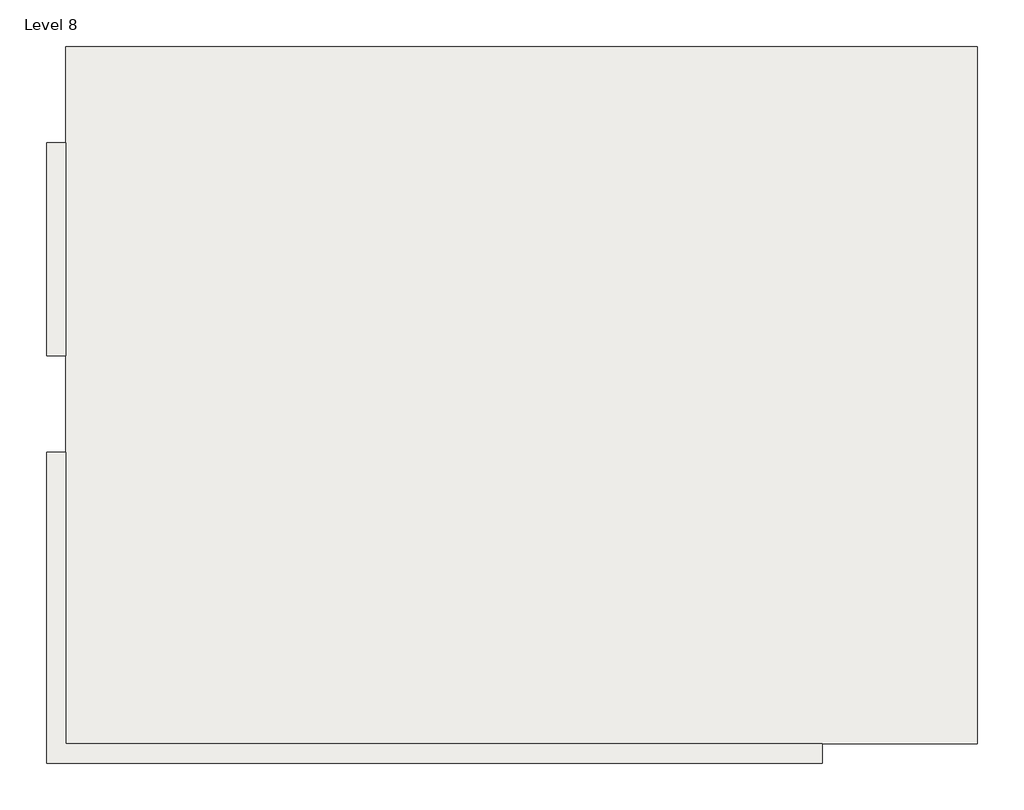
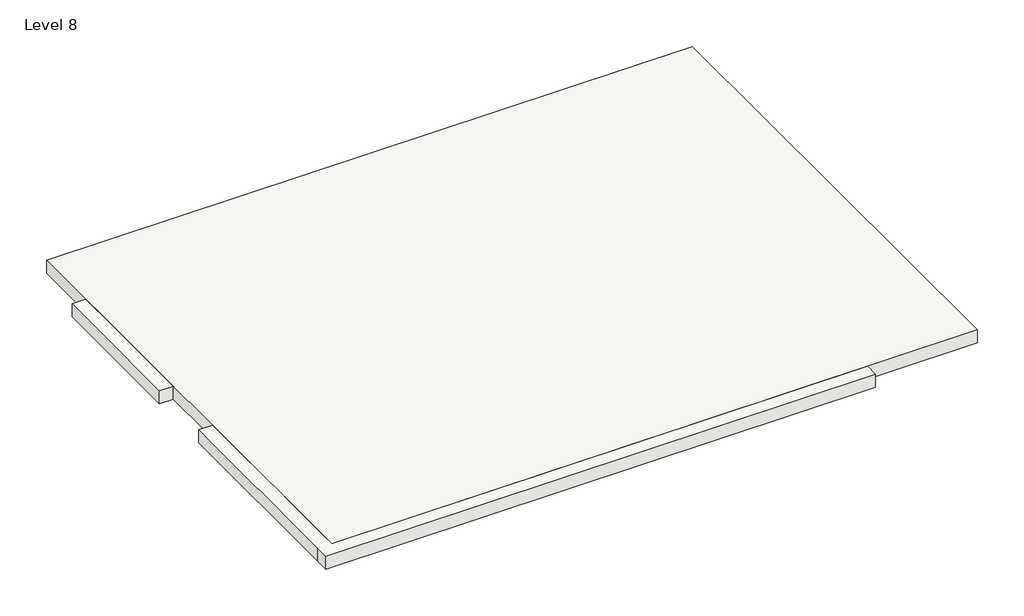
# One storey: 2 slabs.
"""IFC4 building model written with IfcOpenShell, lengths in millimetres."""

from ifc_helpers import new_model, si_unit, frame, origin, place, context, project, spatial, polyline, outline, extrude, element, save

model = new_model("IFC4")

# Units and contexts
model_context = context("Model", 3, world=origin())
ifc_project = project(units=[si_unit("LENGTHUNIT", "METRE", prefix="MILLI")], contexts=[model_context])

# Site, building, storey
site = spatial("IfcSite", under=ifc_project)
building = spatial("IfcBuilding", under=site)
storey = spatial("IfcBuildingStorey", under=building, Name="Level 8", Elevation=21336.0)

# Slabs
placement = place(None, origin())
element("IfcSlab", 1, ObjectType="Generic - 12\"", at=placement, inside=storey, context=model_context, shape_type="SweptSolid", body=[
    extrude(outline(polyline([(-18633.6169582, -41.6299243), (-18328.8169582, -41.6299243), (-18328.8169582, -3394.4299243), (-18633.6169582, -3394.4299243), (-18633.6169582, -41.6299243)])), frame((0.0, 0.0, 19812.0), z_axis=(0.0, 0.0, 1.0), x_axis=(1.0, 0.0, 0.0)), (0.0, 0.0, 1.0), 304.8),
    extrude(outline(polyline([(-18633.6169582, -4908.9117616), (-18328.8169582, -4908.9117616), (-18328.8169582, -9487.2617616), (-6444.7919582, -9487.2617616), (-6444.7919582, -9792.0617616), (-18633.6169582, -9792.0617616), (-18633.6169582, -9487.2617616), (-18633.6169582, -4908.9117616)])), frame((0.0, 0.0, 19812.0), z_axis=(0.0, 0.0, 1.0), x_axis=(1.0, 0.0, 0.0)), (0.0, 0.0, 1.0), 304.8),
])
element("IfcSlab", 2, ObjectType="Generic - 12\" 2", at=placement, inside=storey, context=model_context, shape_type="SweptSolid", body=[
    extrude(outline(polyline([(-4006.3919582, 1466.4882384), (-4006.3919582, -9487.2617616), (-18328.8169582, -9487.2617616), (-18328.8169582, 1466.4882384), (-4006.3919582, 1466.4882384)])), frame((0.0, 0.0, 19812.0), z_axis=(0.0, 0.0, 1.0), x_axis=(1.0, 0.0, 0.0)), (0.0, 0.0, 1.0), 304.8),
])

save(model, "model.ifc")

# Revit data of these elements
# Type "Generic - 12\""
#   Assembly Code = "B1010"
#   Function = 0
#   Layers, outside or top first: 1' - 0" "Parking Stripe" (function 1)
# Type "Generic - 12\" 2"
#   Assembly Code = "B1010"
#   Function = 0
#   Layers, outside or top first: 1' - 0" "Parking Stripe" (function 1)
# Element 1 (IfcSlab, "Generic - 12\"")
#   built-in parameter 1001955 = 3.14159 (stored number, unit not read)
#   Height Offset From Level = -4' - 0"
#   Phase Created = New Construction
#   Materials on its faces: "Parking Stripe"
# Element 2 (IfcSlab, "Generic - 12\" 2")
#   Height Offset From Level = -4' - 0"
#   Phase Created = New Construction
#   Materials on its faces: "Parking Stripe"
# Materials
#   "Parking Stripe": class "Paint", colour RGB 250 250 91, transparency 0, Cost = 0
